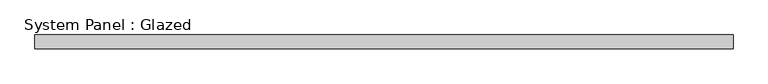
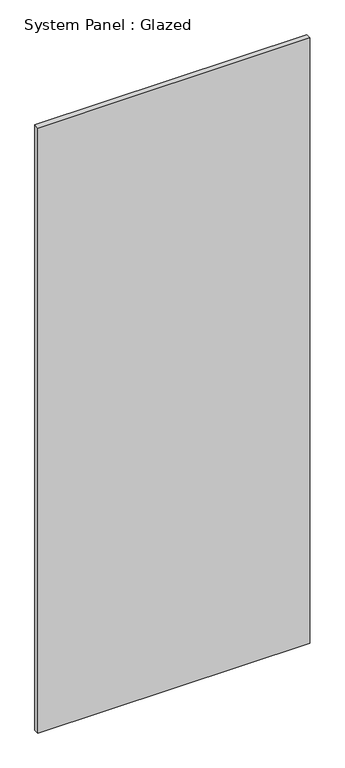
"""IFC4 building model written with IfcOpenShell, lengths in millimetres: plate geometry, System Panel : Glazed."""

from ifc_helpers import new_model, si_unit, origin, origin_with_axes, place, context, project, spatial, polyline, outline, extrude, source, transform, mapped, element, save


def system_panel_glazed_ef83883b(model_context):
    return source(origin(), model_context, "Body", "SweptSolid", [
        extrude(outline(polyline([(637.57, 24.5), (-637.57, 24.5), (-637.57, 49.5), (637.57, 49.5), (637.57, 24.5)])), origin_with_axes(), (0.0, 0.0, 1.0), 3000.0),
    ])


if __name__ == "__main__":
    model = new_model("IFC4")
    model_context = context("Model", 3, world=origin())
    ifc_project = project(units=[si_unit("LENGTHUNIT", "METRE", prefix="MILLI")], contexts=[model_context])
    site = spatial("IfcSite", under=ifc_project)
    building = spatial("IfcBuilding", under=site)
    placement = place(None, origin())
    system_panel_glazed_shape = system_panel_glazed_ef83883b(model_context)
    element("IfcPlate", 1, ObjectType="System Panel : Glazed", at=placement, inside=building, context=model_context, shape_type="MappedRepresentation", body=[
        mapped(system_panel_glazed_shape, transform((0.0, 0.0, 0.0), x_axis=(1.0, 0.0, 0.0), y_axis=(0.0, 1.0, 0.0), z_axis=(0.0, 0.0, 1.0))),
    ])
    save(model, "model.ifc")

# Revit data of these elements
# Type "System Panel : Glazed"
#   Keynote = "H11"
#   Construction Type Id = "GSP4R"
#   Analytic Construction = "1/8 in Pilkington single glazing"
#   Visual Light Transmittance = 0.9
#   Solar Heat Gain Coefficient = 0.86
#   Heat Transfer Coefficient (U) = 6.7069 W/(m²·K)
#   Define Thermal Properties by = 1
# Element 1 (IfcPlate, "System Panel : Glazed")
#   Materials on its faces: "Glass"
# Materials
#   "Glass": class "Glass", colour RGB 0 128 192, transparency 0.9, Description = "Soda Lime Glass", Cost = 0
